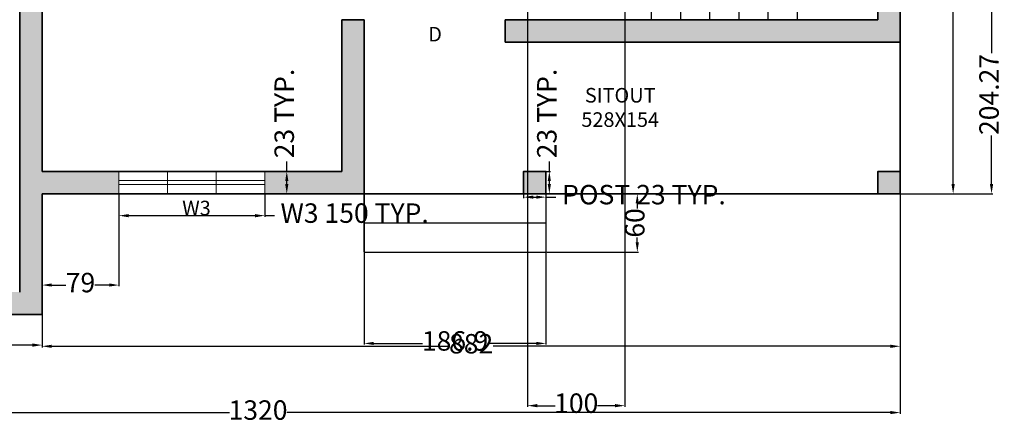
# Model space of a CAD drawing. Units: centimetres. Extents: x 2137 to 3697, y 183 to 2094.
# Tile 3 of 8: x 2685 to 3697, y 183 to 600. Entities that reach past the tile are written whole.
import ezdxf

# ---------------------------------------------------------------- set-up
doc = ezdxf.new("R2010")
doc.units = ezdxf.units.CM
for name, color, linetype, lineweight in [('A-ANNO-DIMS', 2, 'Continuous', 18), ('A-ANNO-TEXT', 7, 'Continuous', 18), ('A-AREA-IDEN', 7, 'Continuous', 25), ('A-COLS', 7, 'Continuous', 35), ('A-FLOR-STRS', 7, 'Continuous', 25), ('A-GLAZ', 4, 'Continuous', 18), ('A-WALL', 7, 'Continuous', 35), ('A-WALL-PATT', 52, 'Continuous', 13)]:
    doc.layers.add(name, color=color, linetype=linetype, lineweight=lineweight)
doc.styles.get("Standard").update_dxf_attribs({"font": 'arial.ttf'})
doc.dimstyles.new('ISO-25', dxfattribs={"dimtxt": 20, "dimasz": 10, "dimexe": 1.25, "dimexo": 0.625, "dimtad": 0, "dimtxsty": 'Standard', "dimcen": 2.5, "dimadec": 0, "dimazin": 0, "dimtfac": 1, "dimtmove": 0, "dimatfit": 3, "dimfxl": 1, "dimarcsym": 0})

# ---------------------------------------------------------------- blocks, each defined once
blk = doc.blocks.new('*D2')
at = {"layer": 'A-ANNO-DIMS', "color": 0, "lineweight": -2, "transparency": 16777216}
for p, q in [((2270, 296), (2270, 263.8)), ((2708, 296), (2708, 263.8)), ((2280, 265), (2465.9, 265)), ((2698, 265), (2512.2, 265))]:
    blk.add_line(p, q, dxfattribs=at)
at = {"layer": 'A-ANNO-DIMS', "color": 0, "transparency": 16777216}
for points in [[(2280, 266.7), (2280, 263.3), (2270, 265)], [(2698, 266.7), (2698, 263.3), (2708, 265)]]:
    blk.add_solid(points, dxfattribs=at)
at = {"layer": 'Defpoints', "color": 0, "transparency": 16777216}
for p in [(2270, 296.6), (2708, 296.6), (2708, 265)]:
    blk.add_point(p, dxfattribs=at)
at = {"layer": 'A-ANNO-DIMS', "color": 0, "transparency": 16777216, "insert": (2489, 265), "char_height": 20, "attachment_point": 5}
blk.add_mtext('438', dxfattribs=at)
blk = doc.blocks.new('*D3')
at = {"layer": 'A-ANNO-DIMS', "color": 0, "lineweight": -2, "transparency": 16777216}
for p, q in [((3590.6, 1986.6), (3645.7, 1986.6)), ((3644.4, 1976.6), (3644.4, 1233.1)), ((3644.4, 430.6), (3644.4, 1174)), ((3590.6, 420.6), (3645.7, 420.6))]:
    blk.add_line(p, q, dxfattribs=at)
at = {"layer": 'A-ANNO-DIMS', "color": 0, "transparency": 16777216}
for points in [[(3642.7, 1976.6), (3646.1, 1976.6), (3644.4, 1986.6)], [(3642.7, 430.6), (3646.1, 430.6), (3644.4, 420.6)]]:
    blk.add_solid(points, dxfattribs=at)
at = {"layer": 'Defpoints', "color": 0, "transparency": 16777216}
for p in [(3590, 1986.6), (3644.4, 1986.6), (3590, 420.6)]:
    blk.add_point(p, dxfattribs=at)
at = {"layer": 'A-ANNO-DIMS', "color": 0, "transparency": 16777216, "insert": (3644.4, 1203.6), "char_height": 20, "attachment_point": 5, "rotation": 90}
blk.add_mtext('1566', dxfattribs=at)
blk = doc.blocks.new('*D4')
at = {"layer": 'A-ANNO-DIMS', "color": 0, "lineweight": -2, "transparency": 16777216}
for p, q in [((2708, 420), (2708, 262.5)), ((3590, 420), (3590, 262.5)), ((2718, 263.8), (3126.4, 263.8)), ((3580, 263.8), (3171.7, 263.8))]:
    blk.add_line(p, q, dxfattribs=at)
at = {"layer": 'A-ANNO-DIMS', "color": 0, "transparency": 16777216}
for points in [[(2718, 265.4), (2718, 262.1), (2708, 263.8)], [(3580, 265.4), (3580, 262.1), (3590, 263.8)]]:
    blk.add_solid(points, dxfattribs=at)
at = {"layer": 'Defpoints', "color": 0, "transparency": 16777216}
for p in [(2708, 420.6), (3590, 420.6), (2708, 263.8)]:
    blk.add_point(p, dxfattribs=at)
at = {"layer": 'A-ANNO-DIMS', "color": 0, "transparency": 16777216, "insert": (3149, 263.8), "char_height": 20, "attachment_point": 5}
blk.add_mtext('882', dxfattribs=at)
blk = doc.blocks.new('*D5')
at = {"layer": 'A-ANNO-DIMS', "color": 0, "lineweight": -2, "transparency": 16777216}
for p, q in [((3590, 420), (3590, 194.4)), ((2270, 296), (2270, 194.4)), ((2280, 195.6), (2900.5, 195.6)), ((3580, 195.6), (2959.5, 195.6))]:
    blk.add_line(p, q, dxfattribs=at)
at = {"layer": 'A-ANNO-DIMS', "color": 0, "transparency": 16777216}
for points in [[(2280, 197.3), (2280, 194), (2270, 195.6)], [(3580, 197.3), (3580, 194), (3590, 195.6)]]:
    blk.add_solid(points, dxfattribs=at)
at = {"layer": 'Defpoints', "color": 0, "transparency": 16777216}
for p in [(3590, 420.6), (2270, 296.6), (3590, 195.6)]:
    blk.add_point(p, dxfattribs=at)
at = {"layer": 'A-ANNO-DIMS', "color": 0, "transparency": 16777216, "insert": (2930, 195.6), "char_height": 20, "attachment_point": 5}
blk.add_mtext('1320', dxfattribs=at)
blk = doc.blocks.new('WIN-W3-150CM')
for p, q in [((0, 23), (0, 0)), ((50, 23), (50, 0)), ((100, 23), (100, 0)), ((150, 23), (150, 0)), ((0, 13.5), (150, 13.5)), ((0, 9.5), (150, 9.5))]:
    blk.add_line(p, q)
blk = doc.blocks.new('POST-23X23CM')
blk.add_lwpolyline([(0, 0), (23, 0), (23, 23), (0, 23)], close=True)
blk = doc.blocks.new('*D20')
at = {"layer": 'A-ANNO-DIMS', "color": 0, "lineweight": -2, "transparency": 16777216}
for p, q in [((2787, 420), (2787, 396.8)), ((2937, 420), (2937, 396.8)), ((2797, 398.1), (2927, 398.1)), ((2937, 398.1), (2947, 398.1))]:
    blk.add_line(p, q, dxfattribs=at)
at = {"layer": 'A-ANNO-DIMS', "color": 0, "transparency": 16777216}
for points in [[(2797, 399.7), (2797, 396.4), (2787, 398.1)], [(2927, 399.7), (2927, 396.4), (2937, 398.1)]]:
    blk.add_solid(points, dxfattribs=at)
at = {"layer": 'Defpoints', "color": 0, "transparency": 16777216}
for p in [(2787, 420.6), (2937, 420.6), (2937, 398.1)]:
    blk.add_point(p, dxfattribs=at)
at = {"layer": 'A-ANNO-DIMS', "color": 0, "transparency": 16777216, "insert": (3029.3, 398.1), "char_height": 20, "attachment_point": 5}
blk.add_mtext('W3 150 TYP.', dxfattribs=at)
blk = doc.blocks.new('*D21')
at = {"layer": 'A-ANNO-DIMS', "color": 0, "lineweight": -2, "transparency": 16777216}
for p, q in [((2959.5, 443.6), (2959.5, 453.6)), ((2937.6, 443.6), (2960.8, 443.6)), ((2959.5, 430.6), (2959.5, 433.6)), ((2937.6, 420.6), (2960.8, 420.6))]:
    blk.add_line(p, q, dxfattribs=at)
at = {"layer": 'A-ANNO-DIMS', "color": 0, "transparency": 16777216}
for points in [[(2957.9, 433.6), (2961.2, 433.6), (2959.5, 443.6)], [(2957.9, 430.6), (2961.2, 430.6), (2959.5, 420.6)]]:
    blk.add_solid(points, dxfattribs=at)
at = {"layer": 'Defpoints', "color": 0, "transparency": 16777216}
for p in [(2937, 443.6), (2959.5, 443.6), (2937, 420.6)]:
    blk.add_point(p, dxfattribs=at)
at = {"layer": 'A-ANNO-DIMS', "color": 0, "transparency": 16777216, "insert": (2959.5, 503.1), "char_height": 20, "attachment_point": 5, "rotation": 90}
blk.add_mtext('23 TYP.', dxfattribs=at)
blk = doc.blocks.new('*D30')
at = {"layer": 'A-ANNO-DIMS', "color": 0, "lineweight": -2, "transparency": 16777216}
for p, q in [((3202.9, 420), (3202.9, 415.9)), ((3212.9, 417.1), (3215.9, 417.1)), ((3225.9, 420), (3225.9, 415.9)), ((3225.9, 417.1), (3235.9, 417.1))]:
    blk.add_line(p, q, dxfattribs=at)
at = {"layer": 'A-ANNO-DIMS', "color": 0, "transparency": 16777216}
for points in [[(3212.9, 418.8), (3212.9, 415.5), (3202.9, 417.1)], [(3215.9, 418.8), (3215.9, 415.5), (3225.9, 417.1)]]:
    blk.add_solid(points, dxfattribs=at)
at = {"layer": 'Defpoints', "color": 0, "transparency": 16777216}
for p in [(3202.9, 420.6), (3225.9, 420.6), (3225.9, 417.1)]:
    blk.add_point(p, dxfattribs=at)
at = {"layer": 'A-ANNO-DIMS', "color": 0, "transparency": 16777216, "insert": (3326.6, 417.1), "char_height": 20, "attachment_point": 5}
blk.add_mtext('POST 23 TYP.', dxfattribs=at)
blk = doc.blocks.new('*D31')
at = {"layer": 'A-ANNO-DIMS', "color": 0, "lineweight": -2, "transparency": 16777216}
for p, q in [((3229.4, 443.6), (3229.4, 453.6)), ((3226.5, 443.6), (3230.6, 443.6)), ((3229.4, 430.6), (3229.4, 433.6)), ((3226.5, 420.6), (3230.6, 420.6))]:
    blk.add_line(p, q, dxfattribs=at)
at = {"layer": 'A-ANNO-DIMS', "color": 0, "transparency": 16777216}
for points in [[(3227.7, 433.6), (3231, 433.6), (3229.4, 443.6)], [(3227.7, 430.6), (3231, 430.6), (3229.4, 420.6)]]:
    blk.add_solid(points, dxfattribs=at)
at = {"layer": 'Defpoints', "color": 0, "transparency": 16777216}
for p in [(3225.9, 443.6), (3229.4, 443.6), (3225.9, 420.6)]:
    blk.add_point(p, dxfattribs=at)
at = {"layer": 'A-ANNO-DIMS', "color": 0, "transparency": 16777216, "insert": (3229.4, 503.1), "char_height": 20, "attachment_point": 5, "rotation": 90}
blk.add_mtext('23 TYP.', dxfattribs=at)
blk = doc.blocks.new('*D38')
at = {"layer": 'A-ANNO-DIMS', "color": 0, "lineweight": -2, "transparency": 16777216}
for p, q in [((2857.4, 1986.6), (2174.9, 1986.6)), ((2176.2, 1976.6), (2176.2, 1171.1)), ((2176.2, 306.6), (2176.2, 1112.1)), ((2269.4, 296.6), (2174.9, 296.6))]:
    blk.add_line(p, q, dxfattribs=at)
at = {"layer": 'A-ANNO-DIMS', "color": 0, "transparency": 16777216}
for points in [[(2174.5, 1976.6), (2177.8, 1976.6), (2176.2, 1986.6)], [(2174.5, 306.6), (2177.8, 306.6), (2176.2, 296.6)]]:
    blk.add_solid(points, dxfattribs=at)
at = {"layer": 'Defpoints', "color": 0, "transparency": 16777216}
for p in [(2176.2, 1986.6), (2858, 1986.6), (2270, 296.6)]:
    blk.add_point(p, dxfattribs=at)
at = {"layer": 'A-ANNO-DIMS', "color": 0, "transparency": 16777216, "insert": (2176.2, 1141.6), "char_height": 20, "attachment_point": 5, "rotation": 90}
blk.add_mtext('1690', dxfattribs=at)
blk = doc.blocks.new('*D40')
at = {"layer": 'A-ANNO-DIMS', "color": 0, "lineweight": -2, "transparency": 16777216}
for p, q in [((3207, 1986), (3207, 201.5)), ((3307, 1986), (3307, 201.5)), ((3217, 202.7), (3235.3, 202.7)), ((3297, 202.7), (3278.8, 202.7))]:
    blk.add_line(p, q, dxfattribs=at)
at = {"layer": 'A-ANNO-DIMS', "color": 0, "transparency": 16777216}
for points in [[(3217, 204.4), (3217, 201.1), (3207, 202.7)], [(3297, 204.4), (3297, 201.1), (3307, 202.7)]]:
    blk.add_solid(points, dxfattribs=at)
at = {"layer": 'Defpoints', "color": 0, "transparency": 16777216}
for p in [(3207, 1986.6), (3307, 1986.6), (3307, 202.7)]:
    blk.add_point(p, dxfattribs=at)
at = {"layer": 'A-ANNO-DIMS', "color": 0, "transparency": 16777216, "insert": (3257, 202.7), "char_height": 20, "attachment_point": 5}
blk.add_mtext('100', dxfattribs=at)
blk = doc.blocks.new('*D45')
at = {"layer": 'A-ANNO-DIMS', "color": 0, "lineweight": -2, "transparency": 16777216}
for p, q in [((3590.6, 624.9), (3685.1, 624.9)), ((3683.9, 614.9), (3683.9, 565)), ((3683.9, 430.6), (3683.9, 480.4)), ((3590.6, 420.6), (3685.1, 420.6))]:
    blk.add_line(p, q, dxfattribs=at)
at = {"layer": 'A-ANNO-DIMS', "color": 0, "transparency": 16777216}
for points in [[(3682.2, 614.9), (3685.5, 614.9), (3683.9, 624.9)], [(3682.2, 430.6), (3685.5, 430.6), (3683.9, 420.6)]]:
    blk.add_solid(points, dxfattribs=at)
at = {"layer": 'Defpoints', "color": 0, "transparency": 16777216}
for p in [(3590, 624.9), (3590, 420.6), (3683.9, 420.6)]:
    blk.add_point(p, dxfattribs=at)
at = {"layer": 'A-ANNO-DIMS', "color": 0, "transparency": 16777216, "insert": (3683.9, 522.7), "char_height": 20, "attachment_point": 5, "rotation": 90}
blk.add_mtext('204.27', dxfattribs=at)
blk = doc.blocks.new('*D54')
at = {"layer": 'A-ANNO-DIMS', "color": 0, "lineweight": -2, "transparency": 16777216}
for p, q in [((2708, 420), (2708, 325.5)), ((2787, 420), (2787, 325.5)), ((2718, 326.7), (2732.6, 326.7)), ((2777, 326.7), (2762.4, 326.7))]:
    blk.add_line(p, q, dxfattribs=at)
at = {"layer": 'A-ANNO-DIMS', "color": 0, "transparency": 16777216}
for points in [[(2718, 328.4), (2718, 325.1), (2708, 326.7)], [(2777, 328.4), (2777, 325.1), (2787, 326.7)]]:
    blk.add_solid(points, dxfattribs=at)
at = {"layer": 'Defpoints', "color": 0, "transparency": 16777216}
for p in [(2708, 420.6), (2787, 420.6), (2708, 326.7)]:
    blk.add_point(p, dxfattribs=at)
at = {"layer": 'A-ANNO-DIMS', "color": 0, "transparency": 16777216, "insert": (2747.5, 326.7), "char_height": 20, "attachment_point": 5}
blk.add_mtext('79', dxfattribs=at)
blk = doc.blocks.new('*D62')
at = {"layer": 'A-ANNO-DIMS', "color": 0, "lineweight": -2, "transparency": 16777216}
for p, q in [((3039, 360), (3039, 265.5)), ((3225.9, 360), (3225.9, 265.5)), ((3049, 266.7), (3099, 266.7)), ((3215.9, 266.7), (3165.9, 266.7))]:
    blk.add_line(p, q, dxfattribs=at)
at = {"layer": 'A-ANNO-DIMS', "color": 0, "transparency": 16777216}
for points in [[(3049, 268.4), (3049, 265.1), (3039, 266.7)], [(3215.9, 268.4), (3215.9, 265.1), (3225.9, 266.7)]]:
    blk.add_solid(points, dxfattribs=at)
at = {"layer": 'Defpoints', "color": 0, "transparency": 16777216}
for p in [(3039, 360.6), (3225.9, 360.6), (3039, 266.7)]:
    blk.add_point(p, dxfattribs=at)
at = {"layer": 'A-ANNO-DIMS', "color": 0, "transparency": 16777216, "insert": (3132.5, 266.7), "char_height": 20, "attachment_point": 5}
blk.add_mtext('186.9', dxfattribs=at)
blk = doc.blocks.new('*D63')
at = {"layer": 'A-ANNO-DIMS', "color": 0, "lineweight": -2, "transparency": 16777216}
for p, q in [((3226.5, 420.6), (3321, 420.6)), ((3319.8, 410.6), (3319.8, 405.5)), ((3319.8, 370.6), (3319.8, 375.6)), ((3226.5, 360.6), (3321, 360.6))]:
    blk.add_line(p, q, dxfattribs=at)
at = {"layer": 'A-ANNO-DIMS', "color": 0, "transparency": 16777216}
for points in [[(3318.1, 410.6), (3321.4, 410.6), (3319.8, 420.6)], [(3318.1, 370.6), (3321.4, 370.6), (3319.8, 360.6)]]:
    blk.add_solid(points, dxfattribs=at)
at = {"layer": 'Defpoints', "color": 0, "transparency": 16777216}
for p in [(3225.9, 420.6), (3225.9, 360.6), (3319.8, 360.6)]:
    blk.add_point(p, dxfattribs=at)
at = {"layer": 'A-ANNO-DIMS', "color": 0, "transparency": 16777216, "insert": (3319.8, 390.6), "char_height": 20, "attachment_point": 5, "rotation": 90}
blk.add_mtext('60', dxfattribs=at)

msp = doc.modelspace()

# ---------------------------------------------------------------- hatches: boundary and pattern name
at = {"layer": 'A-WALL-PATT'}
h = msp.add_hatch(color=256, dxfattribs=at)
h.dxf.hatch_style = 1
h.paths.add_polyline_path([(2413.023, 1526.579), (2270.023, 1526.579), (2270.023, 1413.579), (2293.023, 1413.579), (2293.023, 1503.579), (2413.023, 1503.579)])
h.paths.add_polyline_path([(2744.523, 1526.579), (2563.023, 1526.579), (2563.023, 1503.579), (2638.023, 1503.579), (2683.023, 1503.579), (2683.023, 1296.579), (2706.023, 1296.579), (2706.023, 1503.579), (2744.523, 1503.579)])
h.paths.add_polyline_path([(2881.023, 1541.602), (2858.023, 1541.602), (2858.023, 1526.579), (2819.523, 1526.579), (2819.523, 1503.579), (2858.023, 1503.579), (2858.023, 1311.579), (2781.023, 1311.579), (2781.023, 1296.579), (2858.023, 1296.579), (2858.023, 1273.579), (2881.023, 1273.579)])
h.paths.add_polyline_path([(3207.023, 1745.579), (2881.023, 1745.579), (2881.023, 1963.579), (2913.523, 1963.579), (2913.523, 1986.579), (2858.023, 1986.579), (2858.023, 1691.602), (2881.023, 1691.602), (2881.023, 1722.579), (3184.023, 1722.579), (3184.023, 1321.579), (3207.023, 1321.579)])
h.paths.add_polyline_path([(3072.523, 1986.579), (2988.523, 1986.579), (2988.523, 1963.579), (3021.023, 1963.579), (3021.023, 1820.579), (3036.023, 1820.579), (3036.023, 1963.579), (3072.523, 1963.579)], flags=17)
h.paths.add_polyline_path([(3207.023, 1986.579), (3147.523, 1986.579), (3147.523, 1963.579), (3184.023, 1963.579), (3184.023, 1845.579), (3207.023, 1845.579)], flags=17)
h.paths.add_polyline_path([(3590.023, 1986.579), (3307.023, 1986.579), (3307.023, 1963.579), (3567.023, 1963.579), (3567.023, 1888.579), (3590.023, 1888.579), (3590.023, 1963.579)])
h.paths.add_polyline_path([(3590.023, 1738.579), (3567.023, 1738.579), (3567.023, 1663.579), (3372.023, 1663.579), (3372.023, 1648.579), (3567.023, 1648.579), (3567.023, 1514.579), (3387.023, 1514.579), (3387.023, 1573.579), (3372.023, 1573.579), (3372.023, 1514.579), (3307.023, 1514.579), (3307.023, 1491.579), (3567.023, 1491.579), (3567.023, 1431.579), (3590.023, 1431.579)])
h.paths.add_polyline_path([(3590.023, 1281.579), (3567.023, 1281.579), (3567.023, 1221.579), (3184.023, 1221.579), (3184.023, 922.579), (3207.023, 922.579), (3207.023, 1198.579), (3567.023, 1198.579), (3567.023, 1055.075), (3590.023, 1055.075)])
h.paths.add_polyline_path([(3590.023, 905.075), (3567.023, 905.075), (3567.023, 774.852), (3590.023, 774.852)])
h.paths.add_polyline_path([(3590.023, 624.852), (3567.023, 624.852), (3567.023, 599.579), (3184.023, 599.579), (3184.023, 576.579), (3590.023, 576.579)])
h.paths.add_polyline_path([(3590.023, 443.579), (3567.023, 443.579), (3567.023, 420.579), (3590.023, 420.579)])
h.paths.add_polyline_path([(3225.908, 443.579), (3202.908, 443.579), (3202.908, 420.579), (3225.908, 420.579)])
h.paths.add_polyline_path([(3039.023, 599.579), (3016.023, 599.579), (3016.023, 443.579), (2937.023, 443.579), (2937.023, 420.579), (3039.023, 420.579)])
h.paths.add_polyline_path([(2787.023, 443.579), (2708.023, 443.579), (2708.023, 850.579), (2685.023, 850.579), (2685.023, 319.579), (2564.023, 319.579), (2564.023, 296.579), (2708.023, 296.579), (2708.023, 420.579), (2787.023, 420.579)])
h.paths.add_polyline_path([(2414.023, 319.579), (2293.023, 319.579), (2293.023, 412.079), (2270.023, 412.079), (2270.023, 296.579), (2414.023, 296.579)])
h.paths.add_polyline_path([(2592.023, 677.579), (2293.023, 677.579), (2293.023, 715.079), (2270.023, 715.079), (2270.023, 562.079), (2293.023, 562.079), (2293.023, 637.079), (2293.023, 654.579), (2592.023, 654.579)])
h.paths.add_polyline_path([(2592.023, 850.579), (2526.773, 850.579), (2526.441, 850.508), (2377.032, 850.508), (2293.023, 850.579), (2293.023, 925.579), (2270.023, 925.579), (2270.023, 790.079), (2293.023, 790.079), (2293.023, 827.579), (2569.023, 827.579), (2569.023, 752.579), (2592.023, 752.579)])
h.paths.add_polyline_path([(2293.023, 1263.579), (2270.023, 1263.579), (2270.023, 1075.579), (2293.023, 1075.579), (2293.023, 1150.579), (2881.023, 1150.579), (2881.023, 1173.579), (2293.023, 1173.579)])

# ---------------------------------------------------------------- linework, layer by layer
at = {"layer": 'A-FLOR-STRS'}
for p, q in [((3334.023, 799.579), (3334.023, 599.579)), ((3364.023, 799.579), (3364.023, 599.579)), ((3394.023, 799.579), (3394.023, 599.579)), ((3424.023, 799.579), (3424.023, 599.579)), ((3454.023, 799.579), (3454.023, 599.579)), ((3484.023, 799.579), (3484.023, 599.579)), ((3225.908, 420.579), (3225.908, 360.579)), ((3039.023, 390.579), (3225.908, 390.579)), ((3039.023, 360.579), (3225.908, 360.579))]:
    msp.add_line(p, q, dxfattribs=at)
at = {"layer": 'A-WALL'}
for p, q in [((3590.023, 1986.579), (3590.023, 420.579)), ((3590.023, 1963.579), (3590.023, 420.579)), ((3567.023, 1198.579), (3567.023, 599.579)), ((2685.023, 850.579), (2685.023, 319.579)), ((2708.023, 850.579), (2708.023, 443.579)), ((3016.023, 599.579), (3039.023, 599.579)), ((3016.023, 599.579), (3016.023, 443.579)), ((3039.023, 599.579), (3039.023, 360.579)), ((3184.023, 599.579), (3184.023, 576.579)), ((3184.023, 599.579), (3567.023, 599.579)), ((3184.023, 576.579), (3590.023, 576.579)), ((2708.023, 443.579), (3016.023, 443.579)), ((2708.023, 420.579), (3590.023, 420.579)), ((2708.023, 420.579), (2708.023, 296.579)), ((2270.023, 296.579), (2708.023, 296.579))]:
    msp.add_line(p, q, dxfattribs=at)

# ---------------------------------------------------------------- block references
at = {"layer": 'A-COLS'}
for p in [(3202.908, 420.579), (3567.023, 420.579)]:
    msp.add_blockref('POST-23X23CM', p, dxfattribs=at)
at = {"layer": 'A-GLAZ'}
msp.add_blockref('WIN-W3-150CM', (2787.023, 420.579), dxfattribs=at)

# ---------------------------------------------------------------- texts
at = {"layer": 'A-ANNO-TEXT', "char_height": 15, "attachment_point": 1}
for s, insert in [('\\pxqc;D', (3087.499, 592.163)), ('\\pxqc;W3', (2842.256, 413.41))]:
    msp.add_mtext_dynamic_manual_height_columns(s, width=48.94887, gutter_width=12.5, heights=[0], dxfattribs=dict(at, insert=insert))
at = {"layer": 'A-AREA-IDEN', "insert": (3277.744, 529.372), "char_height": 15, "attachment_point": 1}
msp.add_mtext_dynamic_manual_height_columns('\\pxqc;SITOUT\\P528X154', width=48.94887, gutter_width=12.5, heights=[0], dxfattribs=at)

# ---------------------------------------------------------------- dimensions: what is measured, and where the dimension line sits
at = {"layer": 'A-ANNO-DIMS'}
for base, p1, p2, angle, override, picture, middle in [((2176.173, 1986.579), (2270.023, 296.579), (2858.023, 1986.579), 90, {"dimdec": 0, "dimlfac": 1, "dimrnd": 0, "dimzin": 0, "dimdsep": 46, "dimlunit": 2}, '*D38', (2176.173, 1141.579)), ((3644.405, 1986.579), (3590.023, 420.579), (3590.023, 1986.579), 90, {"dimclrd": 0, "dimclre": 0, "dimclrt": 0}, '*D3', (3644.405, 1203.579)), ((3683.873, 420.579), (3590.023, 624.852), (3590.023, 420.579), 270, {"dimdec": 2, "dimlfac": 1, "dimrnd": 0, "dimzin": 0, "dimdsep": 46, "dimlunit": 2}, '*D45', (3683.873, 522.716)), ((2708.023, 326.729), (2787.023, 420.579), (2708.023, 420.579), 180, {"dimdec": 0, "dimlfac": 1, "dimrnd": 0, "dimzin": 0, "dimdsep": 46, "dimlunit": 2}, '*D54', (2747.523, 326.729)), ((3319.758, 360.579), (3225.908, 420.579), (3225.908, 360.579), 270, {"dimdec": 0, "dimlfac": 1, "dimrnd": 0, "dimzin": 0, "dimdsep": 46, "dimlunit": 2}, '*D63', (3319.758, 390.579)), ((3039.023, 266.729), (3225.908, 360.579), (3039.023, 360.579), 180, {"dimdec": 1, "dimlfac": 1, "dimrnd": 0, "dimzin": 0, "dimdsep": 46, "dimlunit": 2}, '*D62', (3132.465, 266.729))]:
    dim = msp.add_linear_dim(base=base, p1=p1, p2=p2, angle=angle, dimstyle='ISO-25', override=override, dxfattribs=at)
    dim.commit()
    dim.dimension.update_dxf_attribs({"geometry": picture, "text_midpoint": middle})
for base, p1, p2, override, picture, middle in [((3307.023, 202.729), (3207.023, 1986.579), (3307.023, 1986.579), {"dimdec": 0, "dimlfac": 1, "dimrnd": 0, "dimzin": 0, "dimdsep": 46, "dimlunit": 2}, '*D40', (3257.023, 202.729)), ((3590.023, 195.64), (2270.023, 296.579), (3590.023, 420.579), {"dimclrd": 0, "dimclre": 0, "dimclrt": 0}, '*D5', (2930.023, 195.64)), ((2708.023, 263.764), (3590.023, 420.579), (2708.023, 420.579), {"dimclrd": 0, "dimclre": 0, "dimclrt": 0}, '*D4', (3149.023, 263.764)), ((2708.023, 265.014), (2270.023, 296.579), (2708.023, 296.579), {"dimclrd": 0, "dimclre": 0, "dimclrt": 0}, '*D2', (2489.023, 265.014))]:
    dim = msp.add_linear_dim(base=base, p1=p1, p2=p2, dimstyle='ISO-25', override=override, dxfattribs=at)
    dim.commit()
    dim.dimension.update_dxf_attribs({"geometry": picture, "text_midpoint": middle})
for base, p1, p2, picture, middle in [((2959.523, 443.579), (2937.023, 420.579), (2937.023, 443.579), '*D21', (2959.523, 503.052)), ((3229.358, 443.579), (3225.908, 420.579), (3225.908, 443.579), '*D31', (3229.358, 503.052))]:
    dim = msp.add_linear_dim(base=base, p1=p1, p2=p2, angle=90, text='<> TYP.', dimstyle='ISO-25', override={"dimdec": 0, "dimlfac": 1, "dimrnd": 0, "dimzin": 0, "dimdsep": 46, "dimlunit": 2}, dxfattribs=at)
    dim.commit()
    dim.dimension.update_dxf_attribs({"geometry": picture, "text_midpoint": middle})
for base, p1, p2, text, picture, middle in [((3225.908, 417.129), (3202.908, 420.579), (3225.908, 420.579), 'POST <> TYP.', '*D30', (3326.628, 417.129)), ((2937.023, 398.079), (2787.023, 420.579), (2937.023, 420.579), 'W3 <> TYP.', '*D20', (3029.339, 398.079))]:
    dim = msp.add_linear_dim(base=base, p1=p1, p2=p2, text=text, dimstyle='ISO-25', override={"dimdec": 0, "dimlfac": 1, "dimrnd": 0, "dimzin": 0, "dimdsep": 46, "dimlunit": 2}, dxfattribs=at)
    dim.commit()
    dim.dimension.update_dxf_attribs({"geometry": picture, "text_midpoint": middle})

doc.saveas('drawing.dxf')
